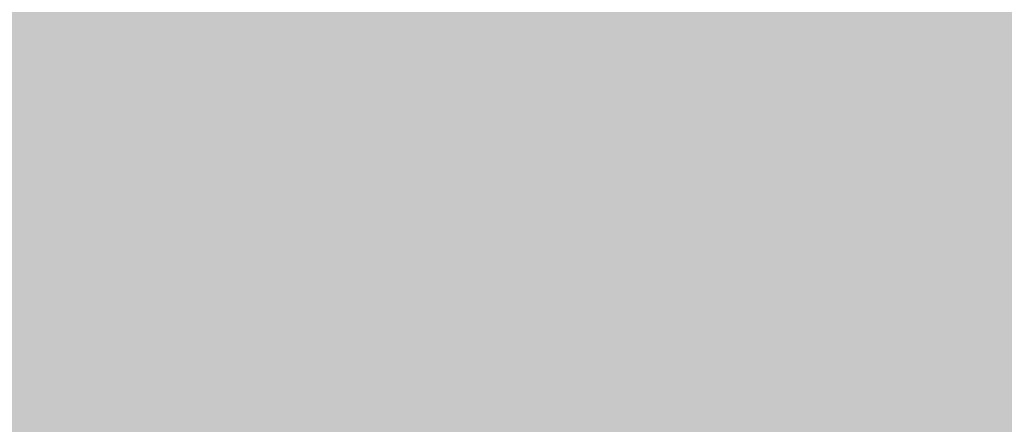
# Model space of a CAD drawing. Units: feet. Extents: x 3168 to 4724, y 827 to 1477.
# Tile 215 of 256: x 3363.87 to 3379.08, y 1087.4 to 1093.65. Entities that reach past the tile are written whole.
import ezdxf

# ---------------------------------------------------------------- set-up
doc = ezdxf.new("R2010")
doc.units = ezdxf.units.FT
doc.layers.add('A-ELEV-PATT', color=8, linetype='Continuous', lineweight=13)

msp = doc.modelspace()

# ---------------------------------------------------------------- hatches: boundary and pattern name
at = {"layer": 'A-ELEV-PATT'}
h = msp.add_hatch(color=256, dxfattribs=at)
h.dxf.hatch_style = 1
edge = h.paths.add_edge_path()
edge.add_ellipse((3552.906, 979.22), major_axis=(36.745, 0), ratio=0.484848, start_angle=0, end_angle=360)
edge = h.paths.add_edge_path()
edge.add_ellipse((3559.892, 929.252), major_axis=(36.745, 0), ratio=0.484848, start_angle=0, end_angle=360)
edge = h.paths.add_edge_path()
edge.add_line((3299.317, 1198.606), (3479.917, 1198.606))
edge.add_line((3479.917, 1198.606), (3479.917, 1209.869))
edge.add_spline(control_points=[(3479.917, 1209.869), (3464.301, 1209.869), (3448.686, 1209.869), (3410.949, 1209.869), (3388.828, 1209.869), (3355.647, 1209.869), (3344.586, 1209.869), (3327.996, 1209.869), (3322.466, 1209.869), (3314.17, 1209.869), (3311.405, 1209.869), (3307.257, 1209.869), (3305.875, 1209.869), (3303.801, 1209.869), (3303.11, 1209.869), (3302.073, 1209.869), (3301.727, 1209.869), (3301.209, 1209.869), (3301.036, 1209.869), (3300.777, 1209.869), (3300.69, 1209.869), (3300.561, 1209.869), (3300.517, 1209.869), (3300.453, 1209.869), (3300.431, 1209.869), (3300.399, 1209.869), (3300.388, 1209.869), (3300.366, 1209.869), (3300.346, 1209.869), (3300.346, 1209.869), (3300.346, 1209.869), (3300.343, 1209.869), (3300.341, 1209.869), (3300.338, 1209.869), (3300.337, 1209.869), (3300.334, 1209.869), (3300.332, 1209.869), (3300.326, 1209.869), (3300.321, 1209.869), (3300.311, 1209.869), (3300.306, 1209.869), (3300.291, 1209.869), (3300.28, 1209.869), (3300.232, 1209.869), (3300.195, 1209.869), (3299.951, 1209.871), (3299.745, 1209.874), (3299.437, 1209.883), (3299.334, 1209.887), (3299.181, 1209.893), (3299.13, 1209.895), (3298.652, 1209.917), (3298.229, 1209.946), (3297.602, 1210.002), (3297.393, 1210.023), (3297.083, 1210.058), (3296.979, 1210.07), (3296.293, 1210.155), (3295.718, 1210.243), (3294.869, 1210.399), (3294.588, 1210.454), (3294.169, 1210.543), (3294.03, 1210.574), (3291.707, 1211.101), (3289.654, 1211.813), (3285.776, 1213.564), (3283.951, 1214.603), (3280.512, 1216.98), (3278.897, 1218.318), (3276.38, 1220.829), (3275.416, 1221.918), (3274.039, 1223.708), (3273.581, 1224.35), (3273.143, 1225.016)], knot_values=[39.119033, 39.119033, 39.119033, 39.119033, 39.286353, 39.286353, 39.523379, 39.523379, 39.641892, 39.641892, 39.701148, 39.701148, 39.730777, 39.730777, 39.745591, 39.745591, 39.752998, 39.752998, 39.756701, 39.756701, 39.758553, 39.758553, 39.759479, 39.759479, 39.759942, 39.759942, 39.760173, 39.760173, 39.760289, 39.760289, 39.760405, 39.760405, 39.760463, 39.760463, 39.763389, 39.763389, 39.764851, 39.764851, 39.767304, 39.767304, 39.773825, 39.773825, 39.78057, 39.78057, 39.79477, 39.79477, 39.845194, 39.845194, 40.126715, 40.126715, 40.267476, 40.267476, 40.337856, 40.337856, 40.927023, 40.927023, 41.221606, 41.221606, 41.368898, 41.368898, 42.202622, 42.202622, 42.619485, 42.619485, 42.827916, 42.827916, 46.118323, 46.118323, 49.408731, 49.408731, 52.699139, 52.699139, 54.927489, 54.927489, 56.104228, 56.104228, 56.104228, 56.104228], weights=[1, 1, 1, 1, 1, 1, 1, 1, 1, 1, 1, 1, 1, 1, 1, 1, 1, 1, 1, 1, 1, 1, 1, 1, 1, 1, 1, 1, 1, 1, 1, 1, 1, 1, 1, 1, 1, 1, 1, 1, 1, 1, 1, 1, 1, 1, 1, 1, 1, 1, 1, 1, 1, 1, 1, 1, 1, 1, 1, 1, 1, 1, 1, 1, 1, 1, 1, 1, 1, 1, 1, 1, 1, 1], degree=3, periodic=0)
edge.add_line((3273.143, 1225.016), (3273.143, 1099.016))
edge.add_line((3273.143, 1099.016), (3299.317, 1099.016))
edge.add_line((3299.317, 1099.016), (3299.317, 1198.606))
edge = h.paths.add_edge_path()
edge.add_line((3304.758, 1324.158), (3479.917, 1324.158))
edge.add_line((3479.917, 1324.158), (3479.917, 1335.715))
edge.add_line((3479.917, 1335.715), (3269.162, 1335.715))
edge.add_spline(control_points=[(3269.162, 1335.715), (3264.024, 1335.715), (3258.364, 1328.958), (3259.264, 1323.9)], knot_values=[0, 0, 0, 0, 15.412191, 15.412191, 15.412191, 15.412191], degree=3, periodic=0)
edge.add_line((3259.264, 1323.9), (3265.517, 1288.769))
edge.add_line((3265.517, 1288.769), (3275.265, 1261.546))
edge.add_line((3275.265, 1261.546), (3304.758, 1261.546))
edge.add_line((3304.758, 1261.546), (3304.758, 1324.158))
h = msp.add_hatch(color=256, dxfattribs=at)
h.dxf.hatch_style = 1
h.paths.add_polyline_path([(3384.525, 1099.016), (3335.029, 1099.016), (3299.317, 1099.016), (3273.143, 1099.016), (3217.565, 1099.016), (3168.069, 827.116), (3335.029, 827.116)])

doc.saveas('drawing.dxf')
